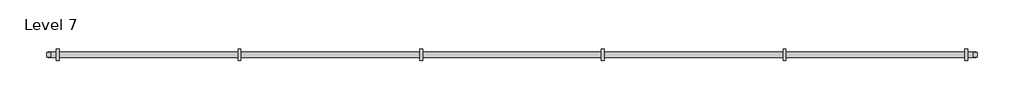
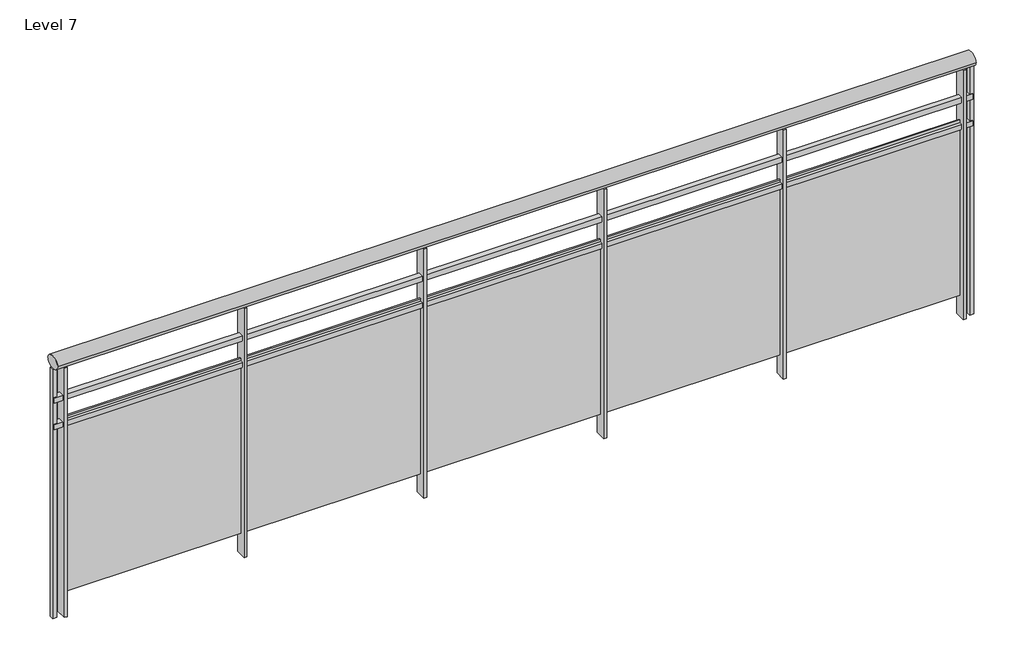
# One storey: 1 railing.
"""IFC4 building model written with IfcOpenShell, lengths in millimetres."""

from ifc_helpers import new_model, si_unit, point, frame, origin, place, context, project, spatial, polyline, ellipse_curve, trimmed, outline, extrude, element, save
from ifc_brep_helpers import plane_surface, extruded_surface, advanced_brep

model = new_model("IFC4")

# Units and contexts
model_context = context("Model", 3, world=origin())
ifc_project = project(units=[si_unit("LENGTHUNIT", "METRE", prefix="MILLI")], contexts=[model_context])

# Site, building, storey
site = spatial("IfcSite", under=ifc_project)
building = spatial("IfcBuilding", under=site)
storey = spatial("IfcBuildingStorey", under=building, Name="Level 7", Elevation=19202.4)

# Railing
placement = place(None, origin())
element("IfcRailing", 1, ObjectType="Glass Panel - Bottom Fill", at=placement, inside=storey, context=model_context, shape_type="SolidModel", body=[
    advanced_brep(
    [(-5729.1673724, -5829.5544725, 20421.6), (-5729.1673724, -5905.7544725, 20421.6), (-1576.8982041, -5829.5544725, 20421.6), (-1576.8982041, -5905.7544725, 20421.6)],
    [
        (0, 1, ellipse_curve(frame((-5729.1673724, -5867.6544725, 20421.6), z_axis=(-1.0, 0.0, 0.0), x_axis=(0.0, -1.0, 0.0)), 38.1, 28.575)),
        (1, 0, ellipse_curve(frame((-5729.1673724, -5867.6544725, 20421.6), z_axis=(-1.0, 0.0, 0.0), x_axis=(0.0, -1.0, 0.0)), 38.1, 28.575)),
        (2, 3, ellipse_curve(frame((-1576.8982041, -5867.6544725, 20421.6), z_axis=(1.0, 0.0, 0.0), x_axis=(0.0, -1.0, 0.0)), 38.1, 28.575)),
        (3, 2, ellipse_curve(frame((-1576.8982041, -5867.6544725, 20421.6), z_axis=(1.0, 0.0, 0.0), x_axis=(0.0, -1.0, 0.0)), 38.1, 28.575)),
        (0, 2),
        (3, 1),
    ],
    [
        plane_surface(frame((-5729.1673724, -5867.6544725, 20421.6), z_axis=(-1.0, 0.0, 0.0), x_axis=(0.0, 1.0, 0.0))),
        plane_surface(frame((-1576.8982041, -5867.6544725, 20421.6), z_axis=(1.0, 0.0, 0.0), x_axis=(0.0, 1.0, 0.0))),
        extruded_surface(trimmed(ellipse_curve(frame((-1576.8982041, -5867.6544725, 20421.6), z_axis=(-1.0, 0.0, 0.0), x_axis=(0.0, -1.0, 0.0)), 38.1, 28.575), [point((-1576.8982041, -5829.5544725, 20421.6))], [point((-1576.8982041, -5905.7544725, 20421.6))], True, "CARTESIAN"), (-4152.2691683, 0.0, 0.0), 4152.2691683),
        extruded_surface(trimmed(ellipse_curve(frame((-1576.8982041, -5867.6544725, 20421.6), z_axis=(-1.0, 0.0, 0.0), x_axis=(0.0, -1.0, 0.0)), 38.1, 28.575), [point((-1576.8982041, -5905.7544725, 20421.6))], [point((-1576.8982041, -5829.5544725, 20421.6))], True, "CARTESIAN"), (-4152.2691683, 0.0, 0.0), 4152.2691683),
    ],
    [
        (0, [[1, 2]]),
        (1, [[3, 4]]),
        (2, [[-1, 5, -4, 6]]),
        (3, [[-2, -6, -3, -5]]),
    ],
),
    extrude(outline(polyline([(-5729.1673724, -5880.3544725), (-5729.1673724, -5854.9544725), (-1576.8982041, -5854.9544725), (-1576.8982041, -5880.3544725), (-5729.1673724, -5880.3544725)])), frame((0.0, 0.0, 20231.1), z_axis=(0.0, 0.0, 1.0), x_axis=(1.0, 0.0, 0.0)), (0.0, 0.0, 1.0), 25.4),
    extrude(outline(polyline([(-5729.1673724, -5880.3544725), (-5729.1673724, -5854.9544725), (-1576.8982041, -5854.9544725), (-1576.8982041, -5880.3544725), (-5729.1673724, -5880.3544725)])), frame((0.0, 0.0, 20104.1), z_axis=(0.0, 0.0, 1.0), x_axis=(1.0, 0.0, 0.0)), (0.0, 0.0, 1.0), 25.4),
    extrude(outline(polyline([(-1627.3827882, -5893.0544725), (-1627.3827882, -5842.2544725), (-1614.6827882, -5842.2544725), (-1614.6827882, -5893.0544725), (-1627.3827882, -5893.0544725)])), frame((0.0, 0.0, 19202.4), z_axis=(0.0, 0.0, 1.0), x_axis=(1.0, 0.0, 0.0)), (0.0, 0.0, 1.0), 1190.625),
    extrude(outline(polyline([(-2433.8327882, -5861.1193155), (-1621.0327882, -5861.1193155), (-1621.0327882, -5867.4693155), (-2433.8327882, -5867.4693155), (-2433.8327882, -5861.1193155)])), frame((0.0, 0.0, 19304.0), z_axis=(0.0, 0.0, 1.0), x_axis=(1.0, 0.0, 0.0)), (0.0, 0.0, 1.0), 838.2),
    extrude(outline(polyline([(-2440.1827882, -5893.0544725), (-2440.1827882, -5842.2544725), (-2427.4827882, -5842.2544725), (-2427.4827882, -5893.0544725), (-2440.1827882, -5893.0544725)])), frame((0.0, 0.0, 19202.4), z_axis=(0.0, 0.0, 1.0), x_axis=(1.0, 0.0, 0.0)), (0.0, 0.0, 1.0), 1190.625),
    extrude(outline(polyline([(-3246.6327882, -5861.1193155), (-2433.8327882, -5861.1193155), (-2433.8327882, -5867.4693155), (-3246.6327882, -5867.4693155), (-3246.6327882, -5861.1193155)])), frame((0.0, 0.0, 19304.0), z_axis=(0.0, 0.0, 1.0), x_axis=(1.0, 0.0, 0.0)), (0.0, 0.0, 1.0), 838.2),
    extrude(outline(polyline([(-3252.9827882, -5893.0544725), (-3252.9827882, -5842.2544725), (-3240.2827882, -5842.2544725), (-3240.2827882, -5893.0544725), (-3252.9827882, -5893.0544725)])), frame((0.0, 0.0, 19202.4), z_axis=(0.0, 0.0, 1.0), x_axis=(1.0, 0.0, 0.0)), (0.0, 0.0, 1.0), 1190.625),
    extrude(outline(polyline([(-4059.4327882, -5861.1193155), (-3246.6327882, -5861.1193155), (-3246.6327882, -5867.4693155), (-4059.4327882, -5867.4693155), (-4059.4327882, -5861.1193155)])), frame((0.0, 0.0, 19304.0), z_axis=(0.0, 0.0, 1.0), x_axis=(1.0, 0.0, 0.0)), (0.0, 0.0, 1.0), 838.2),
    extrude(outline(polyline([(-4065.7827882, -5893.0544725), (-4065.7827882, -5842.2544725), (-4053.0827882, -5842.2544725), (-4053.0827882, -5893.0544725), (-4065.7827882, -5893.0544725)])), frame((0.0, 0.0, 19202.4), z_axis=(0.0, 0.0, 1.0), x_axis=(1.0, 0.0, 0.0)), (0.0, 0.0, 1.0), 1190.625),
    extrude(outline(polyline([(-4872.2327882, -5861.1193155), (-4059.4327882, -5861.1193155), (-4059.4327882, -5867.4693155), (-4872.2327882, -5867.4693155), (-4872.2327882, -5861.1193155)])), frame((0.0, 0.0, 19304.0), z_axis=(0.0, 0.0, 1.0), x_axis=(1.0, 0.0, 0.0)), (0.0, 0.0, 1.0), 838.2),
    extrude(outline(polyline([(-4878.5827882, -5893.0544725), (-4878.5827882, -5842.2544725), (-4865.8827882, -5842.2544725), (-4865.8827882, -5893.0544725), (-4878.5827882, -5893.0544725)])), frame((0.0, 0.0, 19202.4), z_axis=(0.0, 0.0, 1.0), x_axis=(1.0, 0.0, 0.0)), (0.0, 0.0, 1.0), 1190.625),
    extrude(outline(polyline([(-5685.0327882, -5861.1193155), (-4872.2327882, -5861.1193155), (-4872.2327882, -5867.4693155), (-5685.0327882, -5867.4693155), (-5685.0327882, -5861.1193155)])), frame((0.0, 0.0, 19304.0), z_axis=(0.0, 0.0, 1.0), x_axis=(1.0, 0.0, 0.0)), (0.0, 0.0, 1.0), 838.2),
    extrude(outline(polyline([(-5691.3827882, -5893.0544725), (-5691.3827882, -5842.2544725), (-5678.6827882, -5842.2544725), (-5678.6827882, -5893.0544725), (-5691.3827882, -5893.0544725)])), frame((0.0, 0.0, 19202.4), z_axis=(0.0, 0.0, 1.0), x_axis=(1.0, 0.0, 0.0)), (0.0, 0.0, 1.0), 1190.625),
    extrude(outline(polyline([(-1589.5982041, -5877.1794725), (-1589.5982041, -5858.1294725), (-1570.5482041, -5858.1294725), (-1570.5482041, -5877.1794725), (-1589.5982041, -5877.1794725)])), frame((0.0, 0.0, 19202.4), z_axis=(0.0, 0.0, 1.0), x_axis=(1.0, 0.0, 0.0)), (0.0, 0.0, 1.0), 1190.625),
    extrude(outline(polyline([(-5735.5173724, -5877.1794725), (-5735.5173724, -5858.1294725), (-5716.4673724, -5858.1294725), (-5716.4673724, -5877.1794725), (-5735.5173724, -5877.1794725)])), frame((0.0, 0.0, 19202.4), z_axis=(0.0, 0.0, 1.0), x_axis=(1.0, 0.0, 0.0)), (0.0, 0.0, 1.0), 1190.625),
])

save(model, "model.ifc")

# Revit data of these elements
# Type "Glass Panel - Bottom Fill"
#   Assembly Code = "C2010400"
#   built-in parameter 1008612 = 0.0416667 (stored number, unit not read)
#   built-in parameter 1008611 = 0.0416667 (stored number, unit not read)
#   built-in parameter 1008609 = 0.333333 (stored number, unit not read)
#   built-in parameter 1008604 = 0.166667 (stored number, unit not read)
#   built-in parameter 1008603 = 0.166667 (stored number, unit not read)
#   Railing Height = 4' - 0"
#   built-in parameter 1008630 = 2
#   built-in parameter 1008610 = 2
#   built-in parameter 1008618 = Baluster - Square : 3/4"
# Element 1 (IfcRailing, "Glass Panel - Bottom Fill")
#   Phase Created = New Construction
#   Materials on its faces: "Glass"
# Materials
#   "Glass": class "Glass", colour RGB 0 128 192, transparency 0.75, Description = "Soda Lime Glass", Cost = 0
